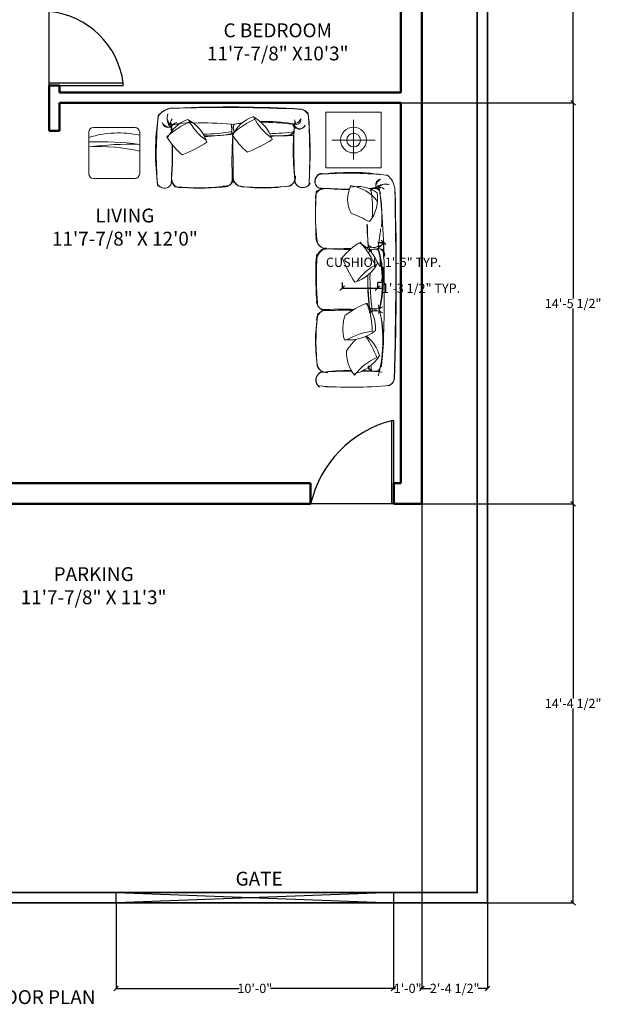
# Model space of a CAD drawing. Units: inches. Extents: x -317284 to 524, y -2236 to 1075.
# Tile 4 of 6: x 273 to 524, y 371 to 796. Entities that reach past the tile are written whole.
import ezdxf

# ---------------------------------------------------------------- set-up
doc = ezdxf.new("R2010")
doc.units = ezdxf.units.IN
doc.header["$MEASUREMENT"] = 0
for name, color, linetype, lineweight in [('A-ANNO-DIMS', 2, 'Continuous', 18), ('A-ANNO-TEXT', 7, 'Continuous', 25), ('A-AREA-IDEN', 7, 'Continuous', 18), ('A-DOOR', 4, 'Continuous', 25), ('A-FURN', 8, 'Continuous', 18), ('A-WALL', 7, 'Continuous', 50), ('C-PROP', 3, 'Continuous', 35), ('C-SITE-GATE', 4, 'Continuous', 25), ('C-SITE-PVMT', 8, 'Continuous', 18)]:
    doc.layers.add(name, color=color, linetype=linetype, lineweight=lineweight)
doc.styles.get("Standard").update_dxf_attribs({"font": 'arial.ttf'})
doc.dimstyles.get("Standard").update_dxf_attribs({"dimtxt": 4, "dimasz": 2, "dimexe": 0.18, "dimexo": 0.0625, "dimgap": 0.09, "dimtad": 0, "dimtih": 1, "dimtoh": 1, "dimdec": 0, "dimzin": 0, "dimdsep": 46, "dimlunit": 4, "dimtxsty": 'Standard', "dimblk": 'OBLIQUE', "dimcen": 0.09, "dimadec": 0, "dimazin": 0, "dimtfac": 1, "dimtdec": 0, "dimtofl": 0, "dimtmove": 0, "dimatfit": 3, "dimldrblk": 'OBLIQUE', "dimfxl": 1, "dimtolj": 1, "dimtzin": 0, "dimarcsym": 0})

# ---------------------------------------------------------------- blocks, each defined once
blk = doc.blocks.new('SDFGHJK')
for p, q in [((282.73, 832.88), (281.73, 832.88)), ((281.73, 832.88), (281.73, 800.88)), ((282.73, 800.88), (282.73, 832.88)), ((282.73, 800.88), (250.73, 800.88))]:
    blk.add_line(p, q)
blk.add_arc((286.22, 797.51), 35.65, 97.2399, 174.5788)
blk = doc.blocks.new('SOFA-CUSHION')
for centre, radius, start, end in [((22.32, -18.36, -275.77), 28.9, 120.3068, 140.5663), ((1.38, -7.28, -275.77), 14.74, 19.4501, 66.7699), ((-21.14, -19.66, -275.77), 39.03, 24.0815, 42.2768), ((57.6, 22.5, -275.77), 61.84, 201.3371, 212.4176), ((0.57, 5.14, -275.77), 16.52, 287.0126, 332.9429), ((24.79, -22.95, -275.77), 22.35, 115.9005, 145.6513)]:
    blk.add_arc(centre, radius, start, end)
blk = doc.blocks.new('_Oblique')
at = {"color": 0, "linetype": 'ByBlock', "lineweight": -2}
blk.add_line((-0.5, -0.5), (0.5, 0.5), dxfattribs=at)
blk = doc.blocks.new('*D19')
at = {"layer": 'A-ANNO-DIMS', "color": 0, "lineweight": -2, "transparency": 16777216}
for p, q in [((427.74, 700.13), (430.44, 700.13)), ((430.26, 700.13), (430.26, 693.67)), ((430.26, 682.89), (430.26, 689.35)), ((427.74, 682.89), (430.44, 682.89))]:
    blk.add_line(p, q, dxfattribs=at)
at = {"layer": 'Defpoints', "color": 0, "transparency": 16777216}
for p in [(427.67, 700.13), (430.26, 700.13), (427.67, 682.89)]:
    blk.add_point(p, dxfattribs=at)
at = {"layer": 'A-ANNO-DIMS', "color": 0, "lineweight": -2, "transparency": 16777216, "xscale": 2, "yscale": 2, "zscale": 2}
for p, rotation in [((430.26, 700.13), 90), ((430.26, 682.89), 270)]:
    blk.add_blockref('_Oblique', p, dxfattribs=dict(at, rotation=rotation))
at = {"layer": 'A-ANNO-DIMS', "color": 0, "transparency": 16777216, "insert": (430.26, 691.51), "char_height": 4, "attachment_point": 5}
blk.add_mtext('\\A1;CUSHION 1\'-5" TYP.', dxfattribs=at)
blk = doc.blocks.new('*D20')
at = {"layer": 'A-ANNO-DIMS', "color": 0, "lineweight": -2, "transparency": 16777216}
for p, q in [((412.4, 682.82), (412.4, 680.12)), ((427.67, 682.82), (427.67, 680.12)), ((412.4, 680.3), (427.67, 680.3)), ((427.67, 680.3), (429.67, 680.3))]:
    blk.add_line(p, q, dxfattribs=at)
at = {"layer": 'Defpoints', "color": 0, "transparency": 16777216}
for p in [(412.4, 682.89), (427.67, 682.89), (427.67, 680.3)]:
    blk.add_point(p, dxfattribs=at)
at = {"layer": 'A-ANNO-DIMS', "color": 0, "lineweight": -2, "transparency": 16777216, "xscale": 2, "yscale": 2, "zscale": 2, "rotation": 180}
blk.add_blockref('_Oblique', (412.4, 680.3), dxfattribs=at)
at = {"layer": 'A-ANNO-DIMS', "color": 0, "lineweight": -2, "transparency": 16777216, "xscale": 2, "yscale": 2, "zscale": 2}
blk.add_blockref('_Oblique', (427.67, 680.3), dxfattribs=at)
at = {"layer": 'A-ANNO-DIMS', "color": 0, "transparency": 16777216, "insert": (446.43, 680.3), "char_height": 4, "attachment_point": 5}
blk.add_mtext('\\A1;1\'-3 1/2" TYP.', dxfattribs=at)
blk = doc.blocks.new('*D36')
at = {"layer": 'A-ANNO-DIMS', "color": 0, "lineweight": -2, "transparency": 16777216}
for p, q in [((446.73, 586.97), (446.73, 377.4)), ((475.23, 414.47), (475.23, 377.4)), ((446.73, 377.58), (450.88, 377.58)), ((475.23, 377.58), (471.08, 377.58))]:
    blk.add_line(p, q, dxfattribs=at)
at = {"layer": 'Defpoints', "color": 0, "transparency": 16777216}
for p in [(446.73, 587.03), (475.23, 414.53), (475.23, 377.58)]:
    blk.add_point(p, dxfattribs=at)
at = {"layer": 'A-ANNO-DIMS', "color": 0, "lineweight": -2, "transparency": 16777216, "xscale": 2, "yscale": 2, "zscale": 2, "rotation": 180}
blk.add_blockref('_Oblique', (446.73, 377.58), dxfattribs=at)
at = {"layer": 'A-ANNO-DIMS', "color": 0, "lineweight": -2, "transparency": 16777216, "xscale": 2, "yscale": 2, "zscale": 2}
blk.add_blockref('_Oblique', (475.23, 377.58), dxfattribs=at)
at = {"layer": 'A-ANNO-DIMS', "color": 0, "transparency": 16777216, "insert": (460.98, 377.58), "char_height": 4, "attachment_point": 5}
blk.add_mtext('\\A1;2\'-4 1/2"', dxfattribs=at)
blk = doc.blocks.new('*D37')
at = {"layer": 'A-ANNO-DIMS', "color": 0, "lineweight": -2, "transparency": 16777216}
for p, q in [((446.73, 586.97), (446.73, 377.4)), ((434.59, 414.47), (434.59, 377.4)), ((434.59, 377.58), (435.44, 377.58)), ((446.73, 377.58), (445.88, 377.58))]:
    blk.add_line(p, q, dxfattribs=at)
at = {"layer": 'Defpoints', "color": 0, "transparency": 16777216}
for p in [(446.73, 587.03), (434.59, 414.53), (446.73, 377.58)]:
    blk.add_point(p, dxfattribs=at)
at = {"layer": 'A-ANNO-DIMS', "color": 0, "lineweight": -2, "transparency": 16777216, "xscale": 2, "yscale": 2, "zscale": 2, "rotation": 180}
blk.add_blockref('_Oblique', (434.59, 377.58), dxfattribs=at)
at = {"layer": 'A-ANNO-DIMS', "color": 0, "lineweight": -2, "transparency": 16777216, "xscale": 2, "yscale": 2, "zscale": 2}
blk.add_blockref('_Oblique', (446.73, 377.58), dxfattribs=at)
at = {"layer": 'A-ANNO-DIMS', "color": 0, "transparency": 16777216, "insert": (440.66, 377.58), "char_height": 4, "attachment_point": 5}
blk.add_mtext('\\A1;1\'-0"', dxfattribs=at)
blk = doc.blocks.new('*D39')
at = {"layer": 'A-ANNO-DIMS', "color": 0, "lineweight": -2, "transparency": 16777216}
for p, q in [((437.79, 760.38), (512.36, 760.38)), ((512.18, 760.38), (512.18, 675.86)), ((512.18, 587.03), (512.18, 671.55)), ((446.79, 587.03), (512.36, 587.03))]:
    blk.add_line(p, q, dxfattribs=at)
at = {"layer": 'Defpoints', "color": 0, "transparency": 16777216}
for p in [(437.73, 760.38), (512.18, 760.38), (446.73, 587.03)]:
    blk.add_point(p, dxfattribs=at)
at = {"layer": 'A-ANNO-DIMS', "color": 0, "lineweight": -2, "transparency": 16777216, "xscale": 2, "yscale": 2, "zscale": 2}
for p, rotation in [((512.18, 760.38), 90), ((512.18, 587.03), 270)]:
    blk.add_blockref('_Oblique', p, dxfattribs=dict(at, rotation=rotation))
at = {"layer": 'A-ANNO-DIMS', "color": 0, "transparency": 16777216, "insert": (512.18, 673.7), "char_height": 4, "attachment_point": 5}
blk.add_mtext('\\A1;14\'-5 1/2"', dxfattribs=at)
blk = doc.blocks.new('*D40')
at = {"layer": 'A-ANNO-DIMS', "color": 0, "lineweight": -2, "transparency": 16777216}
for p, q in [((437.79, 944.38), (512.36, 944.38)), ((512.18, 944.38), (512.18, 854.51)), ((512.18, 760.38), (512.18, 850.25)), ((437.79, 760.38), (512.36, 760.38))]:
    blk.add_line(p, q, dxfattribs=at)
at = {"layer": 'Defpoints', "color": 0, "transparency": 16777216}
for p in [(437.73, 944.38), (512.18, 944.38), (437.73, 760.38)]:
    blk.add_point(p, dxfattribs=at)
at = {"layer": 'A-ANNO-DIMS', "color": 0, "lineweight": -2, "transparency": 16777216, "xscale": 2, "yscale": 2, "zscale": 2}
for p, rotation in [((512.18, 944.38), 90), ((512.18, 760.38), 270)]:
    blk.add_blockref('_Oblique', p, dxfattribs=dict(at, rotation=rotation))
at = {"layer": 'A-ANNO-DIMS', "color": 0, "transparency": 16777216, "insert": (512.18, 852.38), "char_height": 4, "attachment_point": 5}
blk.add_mtext('\\A1;15\'-4"', dxfattribs=at)
blk = doc.blocks.new('*D42')
at = {"layer": 'A-ANNO-DIMS', "color": 0, "lineweight": -2, "transparency": 16777216}
for p, q in [((314.59, 414.47), (314.59, 377.4)), ((434.59, 414.47), (434.59, 377.4)), ((314.59, 377.58), (367.82, 377.58)), ((434.59, 377.58), (381.36, 377.58))]:
    blk.add_line(p, q, dxfattribs=at)
at = {"layer": 'Defpoints', "color": 0, "transparency": 16777216}
for p in [(314.59, 414.53), (434.59, 414.53), (434.59, 377.58)]:
    blk.add_point(p, dxfattribs=at)
at = {"layer": 'A-ANNO-DIMS', "color": 0, "lineweight": -2, "transparency": 16777216, "xscale": 2, "yscale": 2, "zscale": 2, "rotation": 180}
blk.add_blockref('_Oblique', (314.59, 377.58), dxfattribs=at)
at = {"layer": 'A-ANNO-DIMS', "color": 0, "lineweight": -2, "transparency": 16777216, "xscale": 2, "yscale": 2, "zscale": 2}
blk.add_blockref('_Oblique', (434.59, 377.58), dxfattribs=at)
at = {"layer": 'A-ANNO-DIMS', "color": 0, "transparency": 16777216, "insert": (374.59, 377.58), "char_height": 4, "attachment_point": 5}
blk.add_mtext('\\A1;10\'-0"', dxfattribs=at)
blk = doc.blocks.new('*D46')
at = {"layer": 'A-ANNO-DIMS', "color": 0, "lineweight": -2, "transparency": 16777216}
for p, q in [((446.79, 587.03), (512.36, 587.03)), ((512.18, 587.03), (512.18, 502.94)), ((512.18, 414.53), (512.18, 498.62)), ((475.29, 414.53), (512.36, 414.53))]:
    blk.add_line(p, q, dxfattribs=at)
at = {"layer": 'Defpoints', "color": 0, "transparency": 16777216}
for p in [(446.73, 587.03), (512.18, 587.03), (475.23, 414.53)]:
    blk.add_point(p, dxfattribs=at)
at = {"layer": 'A-ANNO-DIMS', "color": 0, "lineweight": -2, "transparency": 16777216, "xscale": 2, "yscale": 2, "zscale": 2}
for p, rotation in [((512.18, 587.03), 90), ((512.18, 414.53), 270)]:
    blk.add_blockref('_Oblique', p, dxfattribs=dict(at, rotation=rotation))
at = {"layer": 'A-ANNO-DIMS', "color": 0, "transparency": 16777216, "insert": (512.18, 500.78), "char_height": 4, "attachment_point": 5}
blk.add_mtext('\\A1;14\'-4 1/2"', dxfattribs=at)

msp = doc.modelspace()

# ---------------------------------------------------------------- linework, layer by layer
at = {"layer": 'A-DOOR'}
for p, q in [((434.73, 623.03), (433.73, 623.03)), ((433.73, 623.03), (433.73, 587.03)), ((434.73, 587.03), (434.73, 623.03)), ((434.73, 587.03), (398.73, 587.03))]:
    msp.add_line(p, q, dxfattribs=at)
msp.add_arc((446.1, 575.99), 48.64, 104.7354, 166.8784, dxfattribs=at)
at = {"layer": 'A-FURN'}
for p, q in [((405.26, 732.34, -275.77), (405.26, 756.34, -275.77)), ((405.26, 756.34, -275.77), (429.26, 756.34, -275.77)), ((429.26, 756.34, -275.77), (429.26, 732.34, -275.77)), ((322.82, 749.74, -275.77), (304.82, 749.74, -275.77)), ((417.26, 744.34, -275.77), (417.26, 753.1, -275.77)), ((302.82, 747.74, -275.77), (302.82, 729.74, -275.77)), ((324.82, 729.74, -275.77), (324.82, 747.74, -275.77)), ((309.05, 741.98, -275.77), (309.05, 741.98, -275.77)), ((417.26, 744.34, -275.77), (407.89, 744.34, -275.77)), ((417.26, 744.34, -275.77), (417.26, 735.91, -275.77)), ((417.26, 744.34, -275.77), (426.62, 744.34, -275.77)), ((429.26, 732.34, -275.77), (405.26, 732.34, -275.77)), ((304.82, 727.74, -275.77), (322.82, 727.74, -275.77)), ((402.46, 643.13, -275.77), (402.46, 643.13, -275.77)), ((402.46, 643.13, -275.77), (402.46, 643.13, -275.77)), ((402.63, 645.38, -275.77), (402.63, 645.38, -275.77)), ((419.85, 643.81, -275.77), (419.85, 643.81, -275.77)), ((420.45, 643.75, -275.77), (420.45, 643.75, -275.77))]:
    msp.add_line(p, q, dxfattribs=at)
for radius in [5.58, 2.95]:
    msp.add_circle((417.26, 744.34, -275.77), radius, dxfattribs=at)
for centre, radius, start, end in [((339.4, 750.4, -275.77), 7.81, 83.8792, 147.1093), ((340.05, 748.64, -275.77), 9.56, 98.6549, 138.7104), ((360.92, 43.37, -275.77), 715.07, 87.2697, 91.7875), ((363.36, 213.97, -275.77), 544.69, 86.6876, 92.4329), ((393.43, 752.89, -275.77), 5.05, 31.8817, 73.9672), ((431.02, 738.89, -275.77), 99.37, 170.8079, 188.3514), ((493.52, 738.25, -275.77), 161.51, 174.0627, 184.6253), ((340.41, 754.1, -275.77), 3.72, 154.8715, 246.7247), ((342.61, 753.79, -275.77), 5.88, 161.2473, 221.1348), ((341.07, 751.53, -275.77), 2.97, 137.7203, 204.4461), ((391.31, 754.73, -275.77), 3.35, 271.184, 337.8216), ((392.22, 753.21, -275.77), 2.22, 268.0108, 6.5585), ((390.46, 748.69, -275.77), 10.02, 43.5462, 63.1435), ((218.15, 738.99, -275.77), 180.35, 355.4325, 5.431), ((133.64, 737.41, -275.77), 264.7, 357.3143, 3.933), ((304.82, 747.74, -275.77), 2, 90, 180), ((322.82, 747.74, -275.77), 2, 0, 90), ((337.94, 753.72, -275.77), 3.83, 207.8433, 279.8684), ((337.03, 752.34, -275.77), 2.51, 189.2916, 317.6289), ((351.6, 651.72, -275.77), 100.26, 92.2017, 98.3067), ((352.52, 630.91, -275.77), 120.85, 95.0871, 96.7491), ((340.9, 749, -275.77), 2.54, 147.7366, 202.2387), ((192.14, 738.78, -275.77), 146.9, 3.7101, 5.0653), ((160.31, 738.14, -275.77), 178.55, 3.1908, 3.7892), ((341.36, 749.16, -275.77), 2.83, 100.6216, 199.193), ((352.52, 630.91, -275.77), 120.85, 84.3639, 92.1219), ((356.38, 749.15, -275.77), 8.25, 344.0479, 14.2061), ((357.95, 749.02, -275.77), 6.78, 351.5362, 18.3493), ((378.17, 659.36, -275.77), 92.68, 95.7795, 98.522), ((368.64, 749.52, -275.77), 3.34, 149.8319, 209.468), ((370.3, 749.76, -275.77), 4.92, 163.3108, 202.6164), ((378.84, 680.39, -275.77), 72.04, 97.803, 100.4557), ((378.84, 680.39, -275.77), 72.04, 79.9466, 91.5903), ((378.17, 659.36, -275.77), 92.68, 82.1551, 90.5585), ((388.67, 749.16, -275.77), 2.94, 276.1174, 43.1189), ((494.33, 739.9, -275.77), 103.15, 172.9836, 187.989), ((390.12, 752.03, -275.77), 1.9, 314.3938, 33.5856), ((622.67, 741.42, -275.77), 231.21, 177.5073, 183.9592), ((394.06, 751.76, -275.77), 2.51, 194.7814, 337.5922), ((393.78, 751.88, -275.77), 2.81, 222.3134, 337.6102), ((315.57, 704.23, -275.77), 43.2, 77.6304, 107.1636), ((350.84, 829.75, -275.77), 82.9, 271.0061, 279.6001), ((351.75, 857.4, -275.77), 111.3, 270.4949, 276.3291), ((350.28, 834.37, -275.77), 88.52, 271.6458, 279.5268), ((374.65, 713, -275.77), 35.41, 105.9625, 107.4638), ((382.55, 918.65, -275.77), 172.54, 263.8872, 264.1215), ((519.22, 735.13, -275.77), 154.5, 175.8425, 183.2873), ((366.77, 748.72, -275.77), 2.1, 209.1313, 222.0141), ((-1761287.91, -30674.5, -275.77), 1761933.09, 1.02115803, 1.02184547), ((519.22, 735.13, -275.77), 154.5, 175.3655, 175.4784), ((378.59, 848.42, -275.77), 101.37, 262.7245, 262.7726), ((378.59, 848.42, -275.77), 101.37, 271.3731, 277.4472), ((382.55, 918.65, -275.77), 172.54, 269.6386, 272.7653), ((379.68, 884.81, -275.77), 138.74, 270.7456, 274.456), ((389.23, 748.75, -275.77), 2.33, 257.6226, 350.3094), ((307.34, 606.77, -275.77), 136.84, 82.6617, 91.8937), ((321.1, 596.57, -275.77), 145.97, 88.539, 97.1936), ((307.36, 661.88, -275.77), 79.64, 77.3313, 93.2642), ((160.31, 738.14, -275.77), 178.55, 355.8027, 1.3803), ((192.14, 738.78, -275.77), 146.9, 354.7422, 1.3335), ((304.82, 729.74, -275.77), 2, 180, 270), ((322.82, 729.74, -275.77), 2, 270, 0), ((370, 729.21, -275.77), 5.21, 186.5867, 283.4511), ((369.03, 728, -275.77), 3.81, 174.9234, 245.6374), ((387.82, 728.51, -275.77), 4.33, 280.9756, 4.9747), ((387.94, 728.11, -275.77), 4.01, 289.8228, 2.4985), ((403.83, 726.55, -275.77), 3.3, 71.3412, 252.8428), ((404.59, 726.27, -275.77), 3.98, 108.7066, 202.6723), ((415.92, 631, -275.77), 99.37, 80.6341, 98.3514), ((415.27, 568.5, -275.77), 161.51, 84.0627, 93.6881), ((427.42, 722.62, -275.77), 7.81, 56.0023, 56.0023), ((425.67, 721.97, -275.77), 9.56, 8.6549, 48.7104), ((335.47, 726.8, -275.77), 3.3, 197.7157, 342.8428), ((335.75, 727.57, -275.77), 3.98, 216.0678, 292.6723), ((342.46, 727.59, -275.77), 3.84, 177.6579, 284.0974), ((341.49, 726.63, -275.77), 2.66, 170.2617, 291.0115), ((349.36, 828.17, -275.77), 104.45, 264.8245, 277.7148), ((350.99, 811.99, -275.77), 88.45, 265.0781, 277.695), ((361.47, 727.45, -275.77), 3.37, 252.9316, 5.1092), ((361.88, 727.69, -275.77), 3.34, 253.4437, 1.8228), ((378.47, 789.5, -275.77), 65.88, 260.0543, 280.4167), ((378.56, 811.79, -275.77), 87.96, 265.2072, 277.551), ((395.34, 727.28, -275.77), 3.54, 194.6379, 334.3095), ((395.34, 727.62, -275.77), 3.77, 213.041, 316.0653), ((427.37, 718.73, -275.77), 12.7, 152.1942, 208.1227), ((418.99, 709.54, -275.77), 14.74, 54.6654, 102.5832), ((413.38, 706.93, -275.77), 17.94, 37.4475, 81.1735), ((426.02, 721.51, -275.77), 2.22, 52.2499, 131.1322), ((429.36, 724.99, -275.77), 2.51, 99.2916, 227.6289), ((430.75, 724.08, -275.77), 3.83, 117.8433, 189.8684), ((430.81, 719.41, -275.77), 5.88, 71.2473, 131.1348), ((428.55, 720.95, -275.77), 2.97, 47.7203, 114.4461), ((431.12, 721.61, -275.77), 3.72, 64.8715, 156.7247), ((370.82, 711.23, -275.77), 58.74, 355.7167, 13.4699), ((489.91, 712.62, -275.77), 89.15, 173.7078, 188.1597), ((404.62, 719.56, -275.77), 3.84, 87.6579, 186.5963), ((576.68, 711.47, -275.77), 175.83, 176.538, 183.2518), ((403.65, 720.53, -275.77), 2.66, 80.2617, 201.0115), ((415.17, 901.71, -275.77), 178.55, 265.8027, 270.0952), ((415.8, 869.88, -275.77), 146.9, 264.7422, 269.8415), ((415.17, 901.71, -275.77), 178.55, 272.8469, 273.7892), ((411.16, 719.22, -275.77), 16.52, 322.2037, 8.1582), ((583.76, 713.43, -275.77), 159.62, 176.6143, 176.7488), ((415.8, 869.88, -275.77), 146.9, 273.3663, 275.0653), ((372.67, 714.52, -275.77), 52.82, 355.9091, 9.3319), ((426.44, 720.94, -275.77), 2.53, 5.5094, 125.3618), ((76, 686.08, -275.77), 354.47, 359.6375, 5.9901), ((-1092.8, 687.62, -275.77), 1528.34, 358.2517, 1.34182), ((-752.3, 685.11, -275.77), 1188.06, 357.87913, 1.76902), ((368.61, 596.98, -275.77), 125.14, 63.6226, 67.6678), ((526.56, 710.53, -275.77), 103.53, 181.5276, 186.7252), ((619.22, 710.24, -275.77), 196.01, 180.6743, 183.6481), ((363.12, 711.21, -275.77), 66.02, 348.572, 355.4817), ((405.77, 702.2, -275.77), 4.77, 180.2562, 250.009), ((406.45, 702.5, -275.77), 5.41, 190.7326, 248.8706), ((426.01, 701, -275.77), 3.13, 213.6302, 319.4072), ((425.98, 701.77, -275.77), 3.86, 229.246, 304.576), ((420.13, 706.47, -275.77), 11.89, 311.3239, 329.6489), ((426.11, 702.34, -275.77), 4.67, 294.9311, 336.316), ((523.24, 685.46, -275.77), 122.32, 175.6872, 184.822), ((408.7, 690.91, -275.77), 7.74, 118.8275, 183.1679), ((406.34, 692.63, -275.77), 5.14, 99.6723, 190.8758), ((523.86, 685.36, -275.77), 122.67, 175.4063, 185.976), ((401.63, 1038.92, -275.77), 341.71, 270.3569, 272.4781), ((420.51, 991.07, -275.77), 294.06, 266.8793, 269.0887), ((401.63, 1038.92, -275.77), 341.71, 273.5599, 273.9253), ((426.25, 694.57, -275.77), 2.7, 42.6233, 153.9248), ((420.51, 991.07, -275.77), 294.06, 270.6475, 270.7982), ((426.38, 693.55, -275.77), 3.6, 58.0934, 131.8441), ((548.21, 683.76, -275.77), 124.8, 173.6313, 174.0106), ((523.2, 684.01, -275.77), 99.73, 172.3637, 172.7445), ((583.76, 713.43, -275.77), 159.62, 185.514, 185.6423), ((534.92, 685.2, -275.77), 110.54, 173.8205, 174.432), ((428.24, 694.91, -275.77), 2.51, 341.7747, 110.1119), ((372.02, 682.94, -275.77), 57.64, 346.4246, 14.6799), ((379.3, 683.26, -275.77), 50.71, 344.5471, 16.7487), ((426.8, 694.1, -275.77), 3.83, 0.3263, 72.3514), ((548.21, 683.76, -275.77), 124.8, 179.0125, 185.4293), ((523.2, 684.01, -275.77), 99.73, 178.887, 188.2861), ((534.92, 685.2, -275.77), 110.54, 179.1949, 187.7065), ((81.41, 675.4, -275.77), 349.15, 355.2123, 1.384), ((404.65, 674.5, -275.77), 3.37, 168.429, 275.1092), ((404.89, 674.09, -275.77), 3.34, 163.4437, 271.8228), ((436.31, 638.72, -275.77), 37.5, 111.2126, 127.0845), ((410.79, 663.1, -275.77), 15.97, 356.0508, 41.5115), ((383.08, 660.47, -275.77), 42.28, 1.5034, 18.4401), ((369.53, 657.8, -275.77), 60.41, 345.2542, 14.7458), ((466.7, 657.5, -275.77), 65.88, 170.0543, 190.4167), ((488.99, 657.41, -275.77), 87.96, 172.0869, 187.551), ((406.41, 665.97, -275.77), 5.21, 96.5867, 173.3659), ((405.2, 666.94, -275.77), 3.81, 103.3965, 179.8407), ((412.33, 516.75, -275.77), 154.5, 88.0798, 93.2873), ((-30997.31, 1762323.88, -275.77), 1761933.09, 271.02119422, 271.02160701), ((428.34, 662.84, -275.77), 15.74, 158.3873, 197.8438), ((426.21, 678.02, -275.77), 6.78, 246.4473, 302.7025), ((390.2, 661.32, -275.77), 35.41, 13.524, 17.4638), ((426.35, 679.59, -275.77), 8.25, 254.0479, 292.8429), ((519.3, 656.92, -275.77), 96.17, 171.1063, 171.8048), ((426.72, 667.33, -275.77), 3.34, 47.9567, 138.0859), ((412.33, 516.75, -275.77), 154.5, 85.3655, 85.3663), ((426.96, 665.67, -275.77), 4.92, 54.1749, 112.4749), ((378.96, 657.48, -275.77), 51.22, 345.3745, 16.5383), ((415.33, 675.8, -275.77), 17.89, 263.6702, 309.5436), ((427.33, 637.45, -275.77), 24.22, 94.7049, 122.2519), ((444.81, 632.51, -275.77), 36.93, 136.0462, 145.9003), ((388.27, 635.87, -275.77), 41.64, 20.3191, 34.4817), ((413.28, 647.12, -275.77), 15.72, 14.8665, 52.3615), ((429.72, 652.46, -275.77), 15.51, 177.2031, 219.1005), ((405.71, 648.15, -275.77), 4.33, 190.9756, 274.9747), ((413.47, 660.4, -275.77), 17.62, 282.4859, 328.3594), ((436.84, 628.46, -275.77), 23.85, 113.5207, 143.4241), ((404.44, 640.64, -275.77), 3.51, 115.1873, 227.995), ((404.81, 640.63, -275.77), 3.77, 113.6813, 233.9016), ((405.31, 648.03, -275.77), 4.01, 199.8228, 272.4985), ((418.61, 413.3, -275.77), 231.21, 90.5455, 93.9592), ((417.1, 541.64, -275.77), 103.15, 90.4744, 97.884), ((418.61, 413.3, -275.77), 231.21, 87.5073, 89.3973), ((417.1, 541.64, -275.77), 103.15, 82.9836, 87.5705), ((562, 656.29, -275.77), 138.74, 183.9965, 184.456), ((519.3, 656.92, -275.77), 96.17, 186.1109, 186.9851), ((426.35, 647.3, -275.77), 2.94, 205.1742, 332.9234), ((425.95, 646.74, -275.77), 2.33, 196.7712, 260.3094), ((525.62, 657.38, -275.77), 101.37, 185.932, 187.4472), ((431.18, 641.92, -275.77), 3.85, 273.9909, 348.3328), ((431.45, 641.41, -275.77), 3.4, 282.8701, 352.7992), ((416.25, 819.56, -275.77), 182.08, 265.5341, 275.2764), ((412.81, 902.33, -275.77), 264.7, 268.2528, 268.8905)]:
    msp.add_arc(centre, radius, start, end, dxfattribs=at)
at = {"layer": 'A-WALL'}
for p, q in [((437.73, 944.38), (437.73, 764.88)), ((446.73, 805.38), (446.73, 587.03)), ((290.23, 767.88), (285.73, 767.88)), ((285.73, 767.88), (285.73, 760.38)), ((290.23, 767.88), (290.23, 764.88)), ((437.73, 764.88), (290.23, 764.88)), ((285.73, 760.38), (285.73, 748.38)), ((437.73, 760.38), (290.23, 760.38)), ((290.23, 748.38), (290.23, 760.38)), ((437.73, 760.38), (437.73, 596.03)), ((285.73, 748.38), (290.23, 748.38)), ((398.73, 596.03), (264.23, 596.03)), ((398.73, 596.03), (398.73, 587.03)), ((437.73, 596.03), (434.73, 596.03)), ((434.73, 596.03), (434.73, 587.03)), ((264.23, 587.03), (398.73, 587.03)), ((434.73, 587.03), (446.73, 587.03))]:
    msp.add_line(p, q, dxfattribs=at)
at = {"layer": 'C-PROP'}
for points in [[(475.23, 1034.38), (475.23, 414.53), (65.73, 414.53), (65.73, 1034.38)], [(470.73, 1029.88), (470.73, 419.03), (70.23, 419.03), (70.23, 1029.88)]]:
    msp.add_lwpolyline(points, close=True, dxfattribs=at)
at = {"layer": 'C-SITE-GATE'}
for p, q in [((314.59, 414.53), (314.59, 419.03)), ((314.59, 419.03), (434.59, 414.53)), ((434.59, 419.03), (314.59, 414.53)), ((434.59, 419.03), (434.59, 414.53))]:
    msp.add_line(p, q, dxfattribs=at)
at = {"layer": 'C-SITE-PVMT'}
msp.add_line((446.73, 587.03), (446.73, 419.03), dxfattribs=at)

# ---------------------------------------------------------------- block references
at = {"layer": 'A-DOOR', "rotation": 270}
msp.add_blockref('SDFGHJK', (-515.15, 1050.61), dxfattribs=at)
at = {"layer": 'A-FURN'}
for p, rotation in [((371.37, 739.18), 90.00000000162113), ((343.18, 737.97), 90.00000000162358)]:
    msp.add_blockref('SOFA-CUSHION', p, dxfattribs=dict(at, rotation=rotation))
msp.add_blockref('SOFA-CUSHION', (412.4, 693.54), dxfattribs=at)

# ---------------------------------------------------------------- texts
at = {"layer": 'A-ANNO-TEXT', "char_height": 6, "attachment_point": 1}
for s, width, insert in [('GATE', 83.0945, (366.29, 428.02)), ('GROUND FLOOR PLAN', 269.2345, (220.89, 376.82))]:
    msp.add_mtext_dynamic_manual_height_columns(s, width=width, gutter_width=30, heights=[0], dxfattribs=dict(at, insert=insert))
at = {"layer": 'A-AREA-IDEN', "char_height": 6, "attachment_point": 1}
for s, width, insert in [('\\pxqc;C BEDROOM \\P11\'7-7/8" X10\'3"', 129.4548, (319.78, 794.78)), ('\\pxqc;LIVING\\P11\'7-7/8" X 12\'0"', 115.1935, (260.83, 714.71)), ('\\pxqc;PARKING\\P11\'7-7/8" X 11\'3"', 100.6596, (254.59, 559.69))]:
    msp.add_mtext_dynamic_manual_height_columns(s, width=width, gutter_width=30, heights=[0], dxfattribs=dict(at, insert=insert))

# ---------------------------------------------------------------- dimensions: what is measured, and where the dimension line sits
at = {"layer": 'A-ANNO-DIMS'}
for base, p1, p2, picture, middle in [((512.18, 944.38), (437.73, 760.38), (437.73, 944.38), '*D40', (512.18, 852.38)), ((512.1766, 760.3794), (446.7266, 587.0289), (437.7266, 760.3794), '*D39', (512.1766, 673.7042)), ((512.18, 587.03), (475.23, 414.53), (446.73, 587.03), '*D46', (512.18, 500.78))]:
    dim = msp.add_linear_dim(base=base, p1=p1, p2=p2, angle=90, dimstyle='Standard', override={"dimdec": 1, "dimlfac": 1, "dimrnd": 0, "dimzin": 1, "dimdsep": 46, "dimlunit": 4, "dimfrac": 2}, dxfattribs=at)
    dim.commit()
    dim.dimension.update_dxf_attribs({"geometry": picture, "text_midpoint": middle})
dim = msp.add_linear_dim(base=(430.26, 700.13), p1=(427.67, 682.89), p2=(427.67, 700.13), angle=90, text='CUSHION <> TYP.', dimstyle='Standard', override={"dimdec": 1, "dimlfac": 1, "dimrnd": 0, "dimzin": 1, "dimdsep": 46, "dimlunit": 4, "dimfrac": 2}, dxfattribs=at)
dim.commit()
dim.dimension.update_dxf_attribs({"geometry": '*D19', "text_midpoint": (430.26, 691.51)})
dim = msp.add_linear_dim(base=(427.67, 680.3), p1=(412.4, 682.89), p2=(427.67, 682.89), text='<> TYP.', dimstyle='Standard', override={"dimdec": 1, "dimlfac": 1, "dimrnd": 0, "dimzin": 1, "dimdsep": 46, "dimlunit": 4, "dimfrac": 2}, dxfattribs=at)
dim.commit()
dim.dimension.update_dxf_attribs({"geometry": '*D20', "text_midpoint": (446.43, 680.3)})
for base, p1, p2, picture, middle in [((446.73, 377.58), (434.59, 414.53), (446.73, 587.03), '*D37', (440.66, 377.58)), ((475.23, 377.58), (446.73, 587.03), (475.23, 414.53), '*D36', (460.98, 377.58)), ((434.59, 377.58), (314.59, 414.53), (434.59, 414.53), '*D42', (374.59, 377.58))]:
    dim = msp.add_linear_dim(base=base, p1=p1, p2=p2, dimstyle='Standard', override={"dimdec": 1, "dimlfac": 1, "dimrnd": 0, "dimzin": 1, "dimdsep": 46, "dimlunit": 4, "dimfrac": 2}, dxfattribs=at)
    dim.commit()
    dim.dimension.update_dxf_attribs({"geometry": picture, "text_midpoint": middle})

doc.saveas('drawing.dxf')
